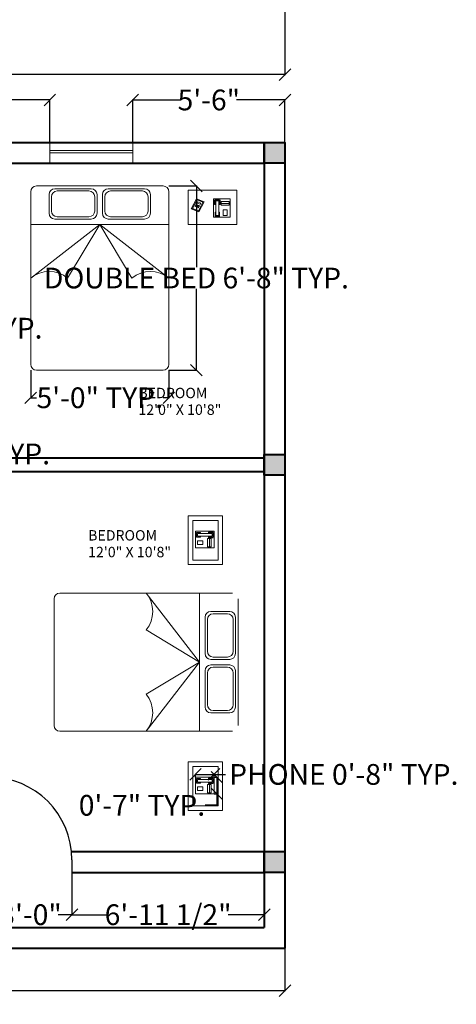
# Model space of a CAD drawing. Units: inches. Extents: x -19 to 1000, y -122 to 1144.
# Tile 5 of 8: x 810 to 1000, y -115 to 313. Entities that reach past the tile are written whole.
import ezdxf

# ---------------------------------------------------------------- set-up
doc = ezdxf.new("R2010")
doc.units = ezdxf.units.IN
doc.header["$MEASUREMENT"] = 0
for name, color, linetype, lineweight in [('A-ANNO-DIMS', 191, 'Continuous', 18), ('A-AREA-IDEN', 1, 'Continuous', 18), ('A-COLS', 4, 'Continuous', 40), ('A-COLS-PATT', 220, 'Continuous', 13), ('A-EQPM', 120, 'Continuous', 18), ('A-FURN-PATT', 254, 'Continuous', 13), ('DOORS', 2, 'Continuous', 25), ('FURNITURE', 120, 'Continuous', 18), ('WALLS', 4, 'Continuous', 40), ('WINDOWS', 3, 'Continuous', 18)]:
    doc.layers.add(name, color=color, linetype=linetype, lineweight=lineweight)
doc.styles.get("Standard").update_dxf_attribs({"font": 'arial.ttf'})
doc.dimstyles.get("Standard").update_dxf_attribs({"dimtxt": 9, "dimasz": 5, "dimexe": 0.18, "dimexo": 0.0625, "dimgap": 0.09, "dimtad": 0, "dimtih": 1, "dimtoh": 1, "dimdec": 0, "dimzin": 0, "dimdsep": 46, "dimlunit": 3, "dimtxsty": 'Standard', "dimblk": 'OBLIQUE', "dimcen": 0.09, "dimadec": 0, "dimazin": 0, "dimtfac": 1, "dimtdec": 0, "dimtofl": 0, "dimtmove": 0, "dimatfit": 3, "dimfxl": 1, "dimtolj": 1, "dimtzin": 0, "dimarcsym": 0})

# ---------------------------------------------------------------- blocks, each defined once
blk = doc.blocks.new('Phone - Desk')
for p, q in [((-4.5, -5), (-4.5, 5)), ((-4.5, 5), (4.5, 5)), ((-4, 4.5), (-4, 2)), ((-4, 2), (-3.25, 2)), ((-3.75, 4.5), (-3.75, 2.25)), ((-1.25, 4.5), (-3.75, 4.5)), ((-3.75, 2.25), (-3.25, 2.25)), ((-3.25, 4), (-3.25, -4)), ((-3.25, 4), (-1.75, 4)), ((-1.75, -4), (-1.75, 4)), ((-1.75, 2.25), (-1.25, 2.25)), ((-1.75, 2), (-1, 2)), ((-1.25, 2.25), (-1.25, 4.5)), ((-1, 2), (-1, 4.5)), ((4, 3.5), (-0.5, 3.5)), ((-0.5, 3.5), (-0.5, 1.5)), ((-0.5, 2.5), (4, 2.5)), ((-0.5, 1.5), (4, 1.5)), ((4, 1.5), (4, 3.5)), ((4.5, 5), (4.5, -5)), ((4.5, -5), (-4.5, -5)), ((-3.75, -2.25), (-3.25, -2.25)), ((-3.75, -4.5), (-3.75, -2.25)), ((-1.25, -4.5), (-3.75, -4.5)), ((-3.25, -4), (-1.75, -4)), ((-1.75, -2.25), (-1.25, -2.25)), ((-1.25, -2.25), (-1.25, -4.5)), ((2.75, -1), (0.75, -1)), ((0.75, -1), (0.75, -4)), ((0.75, -4), (2.75, -4)), ((2.75, -4), (2.75, -1))]:
    blk.add_line(p, q)
blk = doc.blocks.new('*U3')
for p, q in [((0, 0), (0, -6)), ((40, 0), (40, -6))]:
    blk.add_line(p, q)
blk.add_lwpolyline([(0, 0), (0, 40), (1.75, 40), (1.75, 0)], close=True)
blk.add_arc((0, 0), 40, 0, 90)
blk = doc.blocks.new('BED-DOUBLE')
for p, q in [((0, 2.5), (0, 77.5)), ((2.5, 80), (57.5, 80)), ((10.5, 78.8), (26.3, 78.8)), ((11.5, 77.8), (25.3, 77.8)), ((33.7, 78.8), (49.5, 78.8)), ((34.7, 77.8), (48.5, 77.8)), ((60, 77.5), (60, 2.5)), ((8, 68.1), (8, 76.3)), ((9, 69.1), (9, 75.3)), ((27.8, 75.3), (27.8, 69.1)), ((28.8, 76.3), (28.8, 68.1)), ((31.2, 68.1), (31.2, 76.3)), ((32.2, 69.1), (32.2, 75.3)), ((51, 75.3), (51, 69.1)), ((52, 76.3), (52, 68.1)), ((10.5, 65.6), (26.3, 65.6)), ((11.5, 66.6), (25.3, 66.6)), ((33.7, 65.6), (49.5, 65.6)), ((34.7, 66.6), (48.5, 66.6)), ((60, 63.2), (0, 63.2)), ((30, 63.2), (0, 40)), ((30, 63.2), (16.04, 40)), ((30, 63.2), (60, 40)), ((30, 63.2), (43.96, 40)), ((57.5, 0), (2.5, 0))]:
    blk.add_line(p, q)
for centre, radius, start, end in [((2.5, 77.5), 2.5, 90, 180), ((10.5, 76.3), 2.5, 90, 180), ((11.5, 75.3), 2.5, 90, 180), ((25.3, 75.3), 2.5, 0, 90), ((26.3, 76.3), 2.5, 0, 90), ((33.7, 76.3), 2.5, 90, 180), ((34.7, 75.3), 2.5, 90, 180), ((48.5, 75.3), 2.5, 0, 90), ((49.5, 76.3), 2.5, 0, 90), ((57.5, 77.5), 2.5, 0, 90), ((11.5, 69.1), 2.5, 180, 270), ((25.3, 69.1), 2.5, 270, 0), ((34.7, 69.1), 2.5, 180, 270), ((48.5, 69.1), 2.5, 270, 0), ((10.5, 68.1), 2.5, 180, 270), ((26.3, 68.1), 2.5, 270, 0), ((33.7, 68.1), 2.5, 180, 270), ((49.5, 68.1), 2.5, 270, 0), ((8.02, 30.16), 12.7, 50.8272, 129.1728), ((51.98, 30.16), 12.7, 50.8272, 129.1728), ((2.5, 2.5), 2.5, 180, 270), ((57.5, 2.5), 2.5, 270, 0)]:
    blk.add_arc(centre, radius, start, end)
blk = doc.blocks.new('TABLE-BEDSIDE')
for points in [[(0, 0), (21.2, 0), (21.2, 14.94), (0, 14.94)], [(2, 2), (19.2, 2), (19.2, 12.94), (2, 12.94)]]:
    blk.add_lwpolyline(points, close=True)
blk = doc.blocks.new('BOOK-PLAN')
for p, q in [((0, 1.37), (2.34, 5.69)), ((2.34, 5.69), (5.74, 4.34)), ((2.6, 5.21), (2.34, 5.69)), ((2.65, 3.83), (2.98, 4.35)), ((2.98, 4.35), (4.3, 3.83)), ((3.43, 0), (5.74, 4.34)), ((0.61, 1.52), (0, 1.37)), ((0, 1.37), (3.43, 0)), ((3.29, 1.76), (1.59, 2.41)), ((3.42, 2.02), (1.72, 2.68)), ((3.6, 2.31), (1.9, 2.97)), ((3.73, 2.58), (2.03, 3.23)), ((2.65, 3.83), (3.97, 3.3)), ((3.97, 3.3), (4.3, 3.83))]:
    blk.add_line(p, q)
blk.add_lwpolyline([(2.6, 5.21), (5.13, 4.2), (3.16, 0.5), (0.61, 1.52)], close=True)
blk = doc.blocks.new('WIN-36-PLAN')
for p, q in [((0, 4.5), (0, 9)), ((0, 9), (0, 0)), ((36, 9), (36, 0)), ((0, 5.5), (36, 5.5)), ((0, 5.5), (36, 5.5)), ((0, 4.5), (36, 4.5))]:
    blk.add_line(p, q)
blk = doc.blocks.new('COLUMN-9X9')
blk.add_lwpolyline([(0, 9), (9, 9), (9, 0), (0, 0)], close=True)
blk = doc.blocks.new('_Oblique')
at = {"color": 0, "linetype": 'ByBlock', "lineweight": -2}
blk.add_line((-0.5, -0.5), (0.5, 0.5), dxfattribs=at)
blk = doc.blocks.new('*D41')
at = {"layer": 'A-ANNO-DIMS', "color": 0, "lineweight": -2, "transparency": 16777216}
for p, q in [((886.49, -15.91), (886.49, -14.59)), ((886.49, -14.77), (894.51, -14.77)), ((894.51, -15.91), (894.51, -14.59)), ((894.51, -14.77), (899.51, -14.77))]:
    blk.add_line(p, q, dxfattribs=at)
at = {"layer": 'Defpoints', "color": 0, "transparency": 16777216}
for p in [(886.49, -15.97), (894.51, -14.77), (894.51, -15.97)]:
    blk.add_point(p, dxfattribs=at)
at = {"layer": 'A-ANNO-DIMS', "color": 0, "lineweight": -2, "transparency": 16777216, "xscale": 5, "yscale": 5, "zscale": 5, "rotation": 180}
blk.add_blockref('_Oblique', (886.49, -14.77), dxfattribs=at)
at = {"layer": 'A-ANNO-DIMS', "color": 0, "lineweight": -2, "transparency": 16777216, "xscale": 5, "yscale": 5, "zscale": 5}
blk.add_blockref('_Oblique', (894.51, -14.77), dxfattribs=at)
at = {"layer": 'A-ANNO-DIMS', "color": 0, "transparency": 16777216, "insert": (950.91, -14.77), "char_height": 9, "attachment_point": 5}
blk.add_mtext('\\A1;PHONE 0\'-8" TYP.', dxfattribs=at)
blk = doc.blocks.new('*D42')
at = {"layer": 'A-ANNO-DIMS', "color": 0, "lineweight": -2, "transparency": 16777216}
for p, q in [((894.57, -15.97), (895.89, -15.97)), ((895.71, -15.97), (895.71, -23.19)), ((894.57, -23.19), (895.89, -23.19)), ((895.71, -23.19), (895.71, -28.19)), ((895.71, -28.19), (890.71, -28.19))]:
    blk.add_line(p, q, dxfattribs=at)
at = {"layer": 'Defpoints', "color": 0, "transparency": 16777216}
for p in [(894.51, -15.97), (894.51, -23.19), (895.71, -23.19)]:
    blk.add_point(p, dxfattribs=at)
at = {"layer": 'A-ANNO-DIMS', "color": 0, "lineweight": -2, "transparency": 16777216, "xscale": 5, "yscale": 5, "zscale": 5}
for p, rotation in [((895.71, -15.97), 90), ((895.71, -23.19), 270)]:
    blk.add_blockref('_Oblique', p, dxfattribs=dict(at, rotation=rotation))
at = {"layer": 'A-ANNO-DIMS', "color": 0, "transparency": 16777216, "insert": (863.19, -28.19), "char_height": 9, "attachment_point": 5}
blk.add_mtext('\\A1;0\'-7" TYP.', dxfattribs=at)
blk = doc.blocks.new('*D47')
at = {"layer": 'A-ANNO-DIMS', "color": 0, "lineweight": -2, "transparency": 16777216}
for p, q in [((874.92, 240.79), (887.04, 240.79)), ((886.86, 240.79), (886.86, 205.54)), ((886.86, 160.79), (886.86, 196.04)), ((874.92, 160.79), (887.04, 160.79))]:
    blk.add_line(p, q, dxfattribs=at)
at = {"layer": 'Defpoints', "color": 0, "transparency": 16777216}
for p in [(874.86, 240.79), (886.86, 240.79), (874.86, 160.79)]:
    blk.add_point(p, dxfattribs=at)
at = {"layer": 'A-ANNO-DIMS', "color": 0, "lineweight": -2, "transparency": 16777216, "xscale": 5, "yscale": 5, "zscale": 5}
for p, rotation in [((886.86, 240.79), 90), ((886.86, 160.79), 270)]:
    blk.add_blockref('_Oblique', p, dxfattribs=dict(at, rotation=rotation))
at = {"layer": 'A-ANNO-DIMS', "color": 0, "transparency": 16777216, "insert": (886.86, 200.79), "char_height": 9, "attachment_point": 5}
blk.add_mtext('\\A1;DOUBLE BED 6\'-8" TYP.', dxfattribs=at)
blk = doc.blocks.new('*D48')
at = {"layer": 'A-ANNO-DIMS', "color": 0, "lineweight": -2, "transparency": 16777216}
for p, q in [((814.86, 160.73), (814.86, 148.61)), ((874.86, 160.73), (874.86, 148.61)), ((814.86, 148.79), (817.34, 148.79)), ((874.86, 148.79), (872.38, 148.79))]:
    blk.add_line(p, q, dxfattribs=at)
at = {"layer": 'Defpoints', "color": 0, "transparency": 16777216}
for p in [(814.86, 160.79), (874.86, 160.79), (874.86, 148.79)]:
    blk.add_point(p, dxfattribs=at)
at = {"layer": 'A-ANNO-DIMS', "color": 0, "lineweight": -2, "transparency": 16777216, "xscale": 5, "yscale": 5, "zscale": 5, "rotation": 180}
blk.add_blockref('_Oblique', (814.86, 148.79), dxfattribs=at)
at = {"layer": 'A-ANNO-DIMS', "color": 0, "lineweight": -2, "transparency": 16777216, "xscale": 5, "yscale": 5, "zscale": 5}
blk.add_blockref('_Oblique', (874.86, 148.79), dxfattribs=at)
at = {"layer": 'A-ANNO-DIMS', "color": 0, "transparency": 16777216, "insert": (844.86, 148.79), "char_height": 9, "attachment_point": 5}
blk.add_mtext('\\A1;5\'-0" TYP.', dxfattribs=at)
blk = doc.blocks.new('*D53')
at = {"layer": 'A-ANNO-DIMS', "color": 0, "lineweight": -2, "transparency": 16777216}
for p, q in [((763.25, 221.01), (775.96, 221.01)), ((775.78, 221.01), (775.78, 183.75)), ((775.78, 137.01), (775.78, 174.26)), ((763.25, 137.01), (775.96, 137.01))]:
    blk.add_line(p, q, dxfattribs=at)
at = {"layer": 'Defpoints', "color": 0, "transparency": 16777216}
for p in [(763.18, 221.01), (775.78, 221.01), (763.18, 137.01)]:
    blk.add_point(p, dxfattribs=at)
at = {"layer": 'A-ANNO-DIMS', "color": 0, "lineweight": -2, "transparency": 16777216, "xscale": 5, "yscale": 5, "zscale": 5}
for p, rotation in [((775.78, 221.01), 90), ((775.78, 137.01), 270)]:
    blk.add_blockref('_Oblique', p, dxfattribs=dict(at, rotation=rotation))
at = {"layer": 'A-ANNO-DIMS', "color": 0, "transparency": 16777216, "insert": (775.78, 179.01), "char_height": 9, "attachment_point": 5}
blk.add_mtext('\\A1;SOFA 7\'-0" TYP.', dxfattribs=at)
blk = doc.blocks.new('*D54')
at = {"layer": 'A-ANNO-DIMS', "color": 0, "lineweight": -2, "transparency": 16777216}
for p, q in [((737.18, 136.94), (737.18, 124.23)), ((763.18, 136.94), (763.18, 124.23)), ((737.18, 124.41), (763.18, 124.41)), ((763.18, 124.41), (768.18, 124.41))]:
    blk.add_line(p, q, dxfattribs=at)
at = {"layer": 'Defpoints', "color": 0, "transparency": 16777216}
for p in [(737.18, 137.01), (763.18, 137.01), (763.18, 124.41)]:
    blk.add_point(p, dxfattribs=at)
at = {"layer": 'A-ANNO-DIMS', "color": 0, "lineweight": -2, "transparency": 16777216, "xscale": 5, "yscale": 5, "zscale": 5, "rotation": 180}
blk.add_blockref('_Oblique', (737.18, 124.41), dxfattribs=at)
at = {"layer": 'A-ANNO-DIMS', "color": 0, "lineweight": -2, "transparency": 16777216, "xscale": 5, "yscale": 5, "zscale": 5}
blk.add_blockref('_Oblique', (763.18, 124.41), dxfattribs=at)
at = {"layer": 'A-ANNO-DIMS', "color": 0, "transparency": 16777216, "insert": (795.78, 124.41), "char_height": 9, "attachment_point": 5}
blk.add_mtext('\\A1;2\'-2" TYP.', dxfattribs=at)
blk = doc.blocks.new('*D103')
at = {"layer": 'A-ANNO-DIMS', "color": 0, "lineweight": -2, "transparency": 16777216}
for p, q in [((564.34, -90.36), (564.34, -108.87)), ((925.34, -90.36), (925.34, -108.87)), ((564.34, -108.69), (729.3, -108.69)), ((925.34, -108.69), (760.39, -108.69))]:
    blk.add_line(p, q, dxfattribs=at)
at = {"layer": 'Defpoints', "color": 0, "transparency": 16777216}
for p in [(564.34, -90.29), (925.34, -90.29), (925.34, -108.69)]:
    blk.add_point(p, dxfattribs=at)
at = {"layer": 'A-ANNO-DIMS', "color": 0, "lineweight": -2, "transparency": 16777216, "xscale": 5, "yscale": 5, "zscale": 5, "rotation": 180}
blk.add_blockref('_Oblique', (564.34, -108.69), dxfattribs=at)
at = {"layer": 'A-ANNO-DIMS', "color": 0, "lineweight": -2, "transparency": 16777216, "xscale": 5, "yscale": 5, "zscale": 5}
blk.add_blockref('_Oblique', (925.34, -108.69), dxfattribs=at)
at = {"layer": 'A-ANNO-DIMS', "color": 0, "transparency": 16777216, "insert": (744.84, -108.69), "char_height": 9, "attachment_point": 5}
blk.add_mtext('\\A1;30\'-1"', dxfattribs=at)
blk = doc.blocks.new('*D107')
at = {"layer": 'A-ANNO-DIMS', "color": 0, "lineweight": -2, "transparency": 16777216}
for p, q in [((734.18, 259.77), (734.18, 278.29)), ((734.18, 278.11), (766.67, 278.11)), ((823.18, 278.11), (790.7, 278.11)), ((823.18, 259.77), (823.18, 278.29))]:
    blk.add_line(p, q, dxfattribs=at)
at = {"layer": 'Defpoints', "color": 0, "transparency": 16777216}
for p in [(823.18, 278.11), (734.18, 259.71), (823.18, 259.71)]:
    blk.add_point(p, dxfattribs=at)
at = {"layer": 'A-ANNO-DIMS', "color": 0, "lineweight": -2, "transparency": 16777216, "xscale": 5, "yscale": 5, "zscale": 5, "rotation": 180}
blk.add_blockref('_Oblique', (734.18, 278.11), dxfattribs=at)
at = {"layer": 'A-ANNO-DIMS', "color": 0, "lineweight": -2, "transparency": 16777216, "xscale": 5, "yscale": 5, "zscale": 5}
blk.add_blockref('_Oblique', (823.18, 278.11), dxfattribs=at)
at = {"layer": 'A-ANNO-DIMS', "color": 0, "transparency": 16777216, "insert": (778.68, 278.11), "char_height": 9, "attachment_point": 5}
blk.add_mtext('\\A1;7\'-5"', dxfattribs=at)
blk = doc.blocks.new('*D108')
at = {"layer": 'A-ANNO-DIMS', "color": 0, "lineweight": -2, "transparency": 16777216}
for p, q in [((859.18, 259.77), (859.18, 278.29)), ((859.18, 278.11), (880.21, 278.11)), ((925.34, 278.11), (904.31, 278.11)), ((925.34, 259.77), (925.34, 278.29))]:
    blk.add_line(p, q, dxfattribs=at)
at = {"layer": 'Defpoints', "color": 0, "transparency": 16777216}
for p in [(925.34, 278.11), (859.18, 259.71), (925.34, 259.71)]:
    blk.add_point(p, dxfattribs=at)
at = {"layer": 'A-ANNO-DIMS', "color": 0, "lineweight": -2, "transparency": 16777216, "xscale": 5, "yscale": 5, "zscale": 5, "rotation": 180}
blk.add_blockref('_Oblique', (859.18, 278.11), dxfattribs=at)
at = {"layer": 'A-ANNO-DIMS', "color": 0, "lineweight": -2, "transparency": 16777216, "xscale": 5, "yscale": 5, "zscale": 5}
blk.add_blockref('_Oblique', (925.34, 278.11), dxfattribs=at)
at = {"layer": 'A-ANNO-DIMS', "color": 0, "transparency": 16777216, "insert": (892.26, 278.11), "char_height": 9, "attachment_point": 5}
blk.add_mtext('\\A1;5\'-6"', dxfattribs=at)
blk = doc.blocks.new('*D109')
at = {"layer": 'A-ANNO-DIMS', "color": 0, "lineweight": -2, "transparency": 16777216}
for p, q in [((796.78, -57.36), (796.78, -75.87)), ((832.78, -57.36), (832.78, -75.87)), ((796.78, -75.69), (802.73, -75.69)), ((832.78, -75.69), (826.83, -75.69))]:
    blk.add_line(p, q, dxfattribs=at)
at = {"layer": 'Defpoints', "color": 0, "transparency": 16777216}
for p in [(796.78, -57.29), (832.78, -57.29), (796.78, -75.69)]:
    blk.add_point(p, dxfattribs=at)
at = {"layer": 'A-ANNO-DIMS', "color": 0, "lineweight": -2, "transparency": 16777216, "xscale": 5, "yscale": 5, "zscale": 5, "rotation": 180}
blk.add_blockref('_Oblique', (796.78, -75.69), dxfattribs=at)
at = {"layer": 'A-ANNO-DIMS', "color": 0, "lineweight": -2, "transparency": 16777216, "xscale": 5, "yscale": 5, "zscale": 5}
blk.add_blockref('_Oblique', (832.78, -75.69), dxfattribs=at)
at = {"layer": 'A-ANNO-DIMS', "color": 0, "transparency": 16777216, "insert": (814.78, -75.69), "char_height": 9, "attachment_point": 5}
blk.add_mtext('\\A1;3\'-0"', dxfattribs=at)
blk = doc.blocks.new('*D110')
at = {"layer": 'A-ANNO-DIMS', "color": 0, "lineweight": -2, "transparency": 16777216}
for p, q in [((832.78, -57.36), (832.78, -75.87)), ((916.34, -57.36), (916.34, -75.87)), ((832.78, -75.69), (848.5, -75.69)), ((916.34, -75.69), (900.62, -75.69))]:
    blk.add_line(p, q, dxfattribs=at)
at = {"layer": 'Defpoints', "color": 0, "transparency": 16777216}
for p in [(832.78, -57.29), (916.34, -57.29), (832.78, -75.69)]:
    blk.add_point(p, dxfattribs=at)
at = {"layer": 'A-ANNO-DIMS', "color": 0, "lineweight": -2, "transparency": 16777216, "xscale": 5, "yscale": 5, "zscale": 5, "rotation": 180}
blk.add_blockref('_Oblique', (832.78, -75.69), dxfattribs=at)
at = {"layer": 'A-ANNO-DIMS', "color": 0, "lineweight": -2, "transparency": 16777216, "xscale": 5, "yscale": 5, "zscale": 5}
blk.add_blockref('_Oblique', (916.34, -75.69), dxfattribs=at)
at = {"layer": 'A-ANNO-DIMS', "color": 0, "transparency": 16777216, "insert": (874.56, -75.69), "char_height": 9, "attachment_point": 5}
blk.add_mtext('\\A1;6\'-11 1/2"', dxfattribs=at)
blk = doc.blocks.new('*D129')
at = {"layer": 'A-ANNO-DIMS', "color": 0, "lineweight": -2, "transparency": 16777216}
for p, q in [((564.34, 328.07), (564.34, 288.95)), ((925.34, 328.07), (925.34, 288.95)), ((564.34, 289.13), (729.3, 289.13)), ((925.34, 289.13), (760.39, 289.13))]:
    blk.add_line(p, q, dxfattribs=at)
at = {"layer": 'Defpoints', "color": 0, "transparency": 16777216}
for p in [(564.34, 328.13), (925.34, 328.13), (925.34, 289.13)]:
    blk.add_point(p, dxfattribs=at)
at = {"layer": 'A-ANNO-DIMS', "color": 0, "lineweight": -2, "transparency": 16777216, "xscale": 5, "yscale": 5, "zscale": 5, "rotation": 180}
blk.add_blockref('_Oblique', (564.34, 289.13), dxfattribs=at)
at = {"layer": 'A-ANNO-DIMS', "color": 0, "lineweight": -2, "transparency": 16777216, "xscale": 5, "yscale": 5, "zscale": 5}
blk.add_blockref('_Oblique', (925.34, 289.13), dxfattribs=at)
at = {"layer": 'A-ANNO-DIMS', "color": 0, "transparency": 16777216, "insert": (744.84, 289.13), "char_height": 9, "attachment_point": 5}
blk.add_mtext('\\A1;30\'-1"', dxfattribs=at)

msp = doc.modelspace()

# ---------------------------------------------------------------- hatches: boundary and pattern name
at = {"layer": 'A-COLS-PATT'}
h = msp.add_hatch(color=256, dxfattribs=at)
h.dxf.hatch_style = 1
h.paths.add_polyline_path([(573.34, 259.71), (564.34, 259.71), (564.34, 250.71), (573.34, 250.71)])
h.paths.add_polyline_path([(656.01, 259.71), (647.01, 259.71), (647.01, 250.71), (656.01, 250.71)])
h.paths.add_polyline_path([(773.81, 259.71), (764.81, 259.71), (764.81, 250.71), (773.81, 250.71)])
h.paths.add_polyline_path([(925.34, 259.71), (916.34, 259.71), (916.34, 250.71), (925.34, 250.71)])
h = msp.add_hatch(color=256, dxfattribs=at)
h.dxf.hatch_style = 1
h.paths.add_polyline_path([(573.34, 168.48), (564.34, 168.48), (564.34, 159.48), (573.34, 159.48)])
h.paths.add_polyline_path([(654.34, 166.71), (648.34, 166.71), (648.34, 160.71), (654.34, 160.71)])
h.paths.add_polyline_path([(573.34, 124.97), (564.34, 124.97), (564.34, 115.97), (573.34, 115.97)])
h.paths.add_polyline_path([(654.34, 122.71), (648.34, 122.71), (648.34, 116.71), (654.34, 116.71)])
h.paths.add_polyline_path([(654.34, 69.8), (648.34, 69.8), (648.34, 63.8), (654.34, 63.8)])
h.paths.add_polyline_path([(772.34, 69.71), (766.34, 69.71), (766.34, 63.71), (772.34, 63.71)])
h.paths.add_polyline_path([(772.34, 122.71), (766.34, 122.71), (766.34, 116.71), (772.34, 116.71)])
h.paths.add_polyline_path([(925.34, 124.12), (916.34, 124.12), (916.34, 115.12), (925.34, 115.12)])
h.paths.add_polyline_path([(925.34, -48.29), (916.34, -48.29), (916.34, -57.29), (925.34, -57.29)])
h.paths.add_polyline_path([(772.34, -48.29), (766.34, -48.29), (766.34, -57.29), (772.34, -57.29)])
h.paths.add_polyline_path([(654.34, -48.29), (648.34, -48.29), (648.34, -57.29), (654.34, -57.29)])
h.paths.add_polyline_path([(573.34, -48.29), (564.34, -48.29), (564.34, -57.29), (573.34, -57.29)])
at = {"layer": 'A-FURN-PATT'}
h = msp.add_hatch(color=256, dxfattribs=at)
h.dxf.hatch_style = 1
h.paths.add_polyline_path([(887.15, 234.74), (886.89, 235.23), (884.55, 230.9), (885.16, 231.05)])
h.paths.add_polyline_path([(890.29, 233.87), (886.89, 235.23), (887.15, 234.74), (889.68, 233.73), (887.71, 230.03), (885.16, 231.05), (884.55, 230.9), (887.98, 229.53)])

# ---------------------------------------------------------------- linework, layer by layer
at = {"layer": 'FURNITURE'}
for p, q in [((825.02, 6.49), (825.02, 61.49)), ((827.52, 63.99), (902.52, 63.99)), ((888.22, 33.99), (865.02, 63.99)), ((888.22, 3.99), (888.22, 63.99)), ((905.02, 61.49), (905.02, 6.49)), ((893.12, 55.99), (901.32, 55.99)), ((890.62, 53.49), (890.62, 37.69)), ((891.62, 52.49), (891.62, 38.69)), ((894.12, 54.99), (900.32, 54.99)), ((902.82, 52.49), (902.82, 38.69)), ((903.82, 53.49), (903.82, 37.69)), ((888.22, 33.99), (865.02, 47.95)), ((901.32, 35.19), (893.12, 35.19)), ((900.32, 36.19), (894.12, 36.19)), ((888.22, 33.99), (865.02, 3.99)), ((888.22, 33.99), (865.02, 20.03)), ((890.62, 30.29), (890.62, 14.49)), ((893.12, 32.79), (901.32, 32.79)), ((894.12, 31.79), (900.32, 31.79)), ((903.82, 30.29), (903.82, 14.49)), ((891.62, 29.29), (891.62, 15.49)), ((902.82, 29.29), (902.82, 15.49)), ((900.32, 12.99), (894.12, 12.99)), ((901.32, 11.99), (893.12, 11.99)), ((902.52, 3.99), (827.52, 3.99))]:
    msp.add_line(p, q, dxfattribs=at)
msp.add_lwpolyline([(883.29, 223.98), (904.49, 223.98), (904.49, 238.92), (883.29, 238.92)], close=True, dxfattribs=at)
for centre, radius, start, end in [((827.52, 61.49), 2.5, 90, 180), ((855.18, 55.97), 12.7, 320.8272, 39.1728), ((893.12, 53.49), 2.5, 90, 180), ((901.32, 53.49), 2.5, 0, 90), ((894.12, 52.49), 2.5, 90, 180), ((900.32, 52.49), 2.5, 0, 90), ((894.12, 38.69), 2.5, 180, 270), ((900.32, 38.69), 2.5, 270, 0), ((893.12, 37.69), 2.5, 180, 270), ((901.32, 37.69), 2.5, 270, 0), ((893.12, 30.29), 2.5, 90, 180), ((894.12, 29.29), 2.5, 90, 180), ((900.32, 29.29), 2.5, 0, 90), ((901.32, 30.29), 2.5, 0, 90), ((855.18, 12.01), 12.7, 320.8272, 39.1728), ((893.12, 14.49), 2.5, 180, 270), ((894.12, 15.49), 2.5, 180, 270), ((900.32, 15.49), 2.5, 270, 0), ((901.32, 14.49), 2.5, 270, 0), ((827.52, 6.49), 2.5, 180, 270)]:
    msp.add_arc(centre, radius, start, end, dxfattribs=at)
at = {"layer": 'WALLS'}
for p, q in [((564.34, 259.71), (925.34, 259.71)), ((916.34, 259.71), (916.34, -81.29)), ((925.34, 259.71), (925.34, -90.29)), ((772.34, 250.71), (916.34, 250.71)), ((772.34, 122.71), (916.34, 122.71)), ((772.34, 116.71), (916.34, 116.71)), ((832.6, -48.29), (916.34, -48.29)), ((832.78, -57.29), (916.34, -57.29)), ((654.34, -81.29), (916.34, -81.29)), ((766.34, -90.29), (925.34, -90.29))]:
    msp.add_line(p, q, dxfattribs=at)

# ---------------------------------------------------------------- block references
at = {"layer": 'A-COLS'}
for p in [(916.34, 250.71), (916.34, 115.12), (916.34, -57.3)]:
    msp.add_blockref('COLUMN-9X9', p, dxfattribs=at)
at = {"layer": 'A-EQPM', "xscale": 0.8015722193121366, "yscale": 0.8015722193121366, "zscale": 0.8015722193121366}
msp.add_blockref('Phone - Desk', (897.95, 231.16), dxfattribs=at)
at = {"layer": 'A-EQPM', "xscale": 0.8015722193121366, "yscale": 0.8015722193121366, "zscale": 0.8015722193121366, "rotation": 270}
for p in [(890.5, 87.24), (890.5, -19.58)]:
    msp.add_blockref('Phone - Desk', p, dxfattribs=at)
at = {"layer": 'DOORS', "xscale": 0.9, "yscale": 0.9, "zscale": 0.9}
msp.add_blockref('*U3', (796.78, -51.89), dxfattribs=at)
at = {"layer": 'FURNITURE'}
for name, p in [('BED-DOUBLE', (814.86, 160.79)), ('BOOK-PLAN', (884.55, 229.53))]:
    msp.add_blockref(name, p, dxfattribs=at)
at = {"layer": 'FURNITURE', "rotation": 269.9999999999998}
for p in [(883.32, 97.54), (883.32, -9.28)]:
    msp.add_blockref('TABLE-BEDSIDE', p, dxfattribs=at)
at = {"layer": 'WINDOWS'}
msp.add_blockref('WIN-36-PLAN', (823.18, 250.71), dxfattribs=at)

# ---------------------------------------------------------------- texts
at = {"layer": 'A-AREA-IDEN'}
for s, height, p in [('BEDROOM', 4.516, (861.64, 148.61)), ('12\'0" X 10\'8"', 4.5155, (861.64, 141.36)), ('BEDROOM', 4.516, (839.79, 86.8)), ('12\'0" X 10\'8"', 4.5155, (839.79, 79.54))]:
    msp.add_text(s, height=height, dxfattribs=at).set_placement(p)

# ---------------------------------------------------------------- dimensions: what is measured, and where the dimension line sits
at = {"layer": 'A-ANNO-DIMS'}
for base, p1, p2, picture, middle in [((925.34, 289.13), (564.34, 328.13), (925.34, 328.13), '*D129', (744.84, 289.13)), ((823.18, 278.11), (734.18, 259.71), (823.18, 259.71), '*D107', (778.68, 278.11)), ((925.34, 278.11), (859.18, 259.71), (925.34, 259.71), '*D108', (892.26, 278.11)), ((925.34, -108.69), (564.34, -90.29), (925.34, -90.29), '*D103', (744.84, -108.69))]:
    dim = msp.add_linear_dim(base=base, p1=p1, p2=p2, dimstyle='Standard', override={"dimdec": 1, "dimlfac": 1, "dimrnd": 0, "dimzin": 1, "dimdsep": 46, "dimlunit": 4, "dimfrac": 2}, dxfattribs=at)
    dim.commit()
    dim.dimension.update_dxf_attribs({"geometry": picture, "text_midpoint": middle})
for base, p1, p2, angle, text, picture, middle in [((886.86, 240.79), (874.86, 160.79), (874.86, 240.79), 90, 'DOUBLE BED <> TYP.', '*D47', (886.86, 200.79)), ((775.78, 221.01), (763.18, 137.01), (763.18, 221.01), 90, 'SOFA <> TYP.', '*D53', (775.78, 179.01)), ((895.71, -23.19), (894.51, -15.97), (894.51, -23.19), 270, '<> TYP.', '*D42', (863.19, -28.19))]:
    dim = msp.add_linear_dim(base=base, p1=p1, p2=p2, angle=angle, text=text, dimstyle='Standard', override={"dimdec": 1, "dimlfac": 1, "dimrnd": 0, "dimzin": 1, "dimdsep": 46, "dimlunit": 4, "dimfrac": 2}, dxfattribs=at)
    dim.commit()
    dim.dimension.update_dxf_attribs({"geometry": picture, "text_midpoint": middle})
for base, p1, p2, text, picture, middle in [((874.86, 148.79), (814.86, 160.79), (874.86, 160.79), '<> TYP.', '*D48', (844.86, 148.79)), ((763.18, 124.41), (737.18, 137.01), (763.18, 137.01), '<> TYP.', '*D54', (795.78, 124.41)), ((894.51, -14.77), (886.49, -15.97), (894.51, -15.97), 'PHONE <> TYP.', '*D41', (950.91, -14.77))]:
    dim = msp.add_linear_dim(base=base, p1=p1, p2=p2, text=text, dimstyle='Standard', override={"dimdec": 1, "dimlfac": 1, "dimrnd": 0, "dimzin": 1, "dimdsep": 46, "dimlunit": 4, "dimfrac": 2}, dxfattribs=at)
    dim.commit()
    dim.dimension.update_dxf_attribs({"geometry": picture, "text_midpoint": middle})
for base, p1, p2, picture, middle in [((796.78, -75.69), (832.78, -57.29), (796.78, -57.29), '*D109', (814.78, -75.69)), ((832.78, -75.69), (916.34, -57.29), (832.78, -57.29), '*D110', (874.56, -75.69))]:
    dim = msp.add_linear_dim(base=base, p1=p1, p2=p2, angle=180, dimstyle='Standard', override={"dimdec": 1, "dimlfac": 1, "dimrnd": 0, "dimzin": 1, "dimdsep": 46, "dimlunit": 4, "dimfrac": 2}, dxfattribs=at)
    dim.commit()
    dim.dimension.update_dxf_attribs({"geometry": picture, "text_midpoint": middle})

doc.saveas('drawing.dxf')
